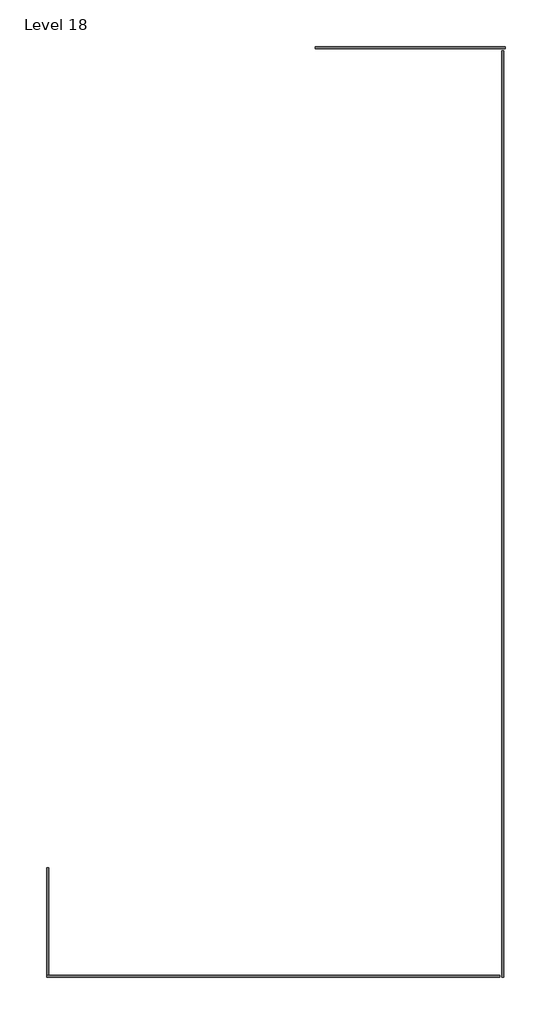
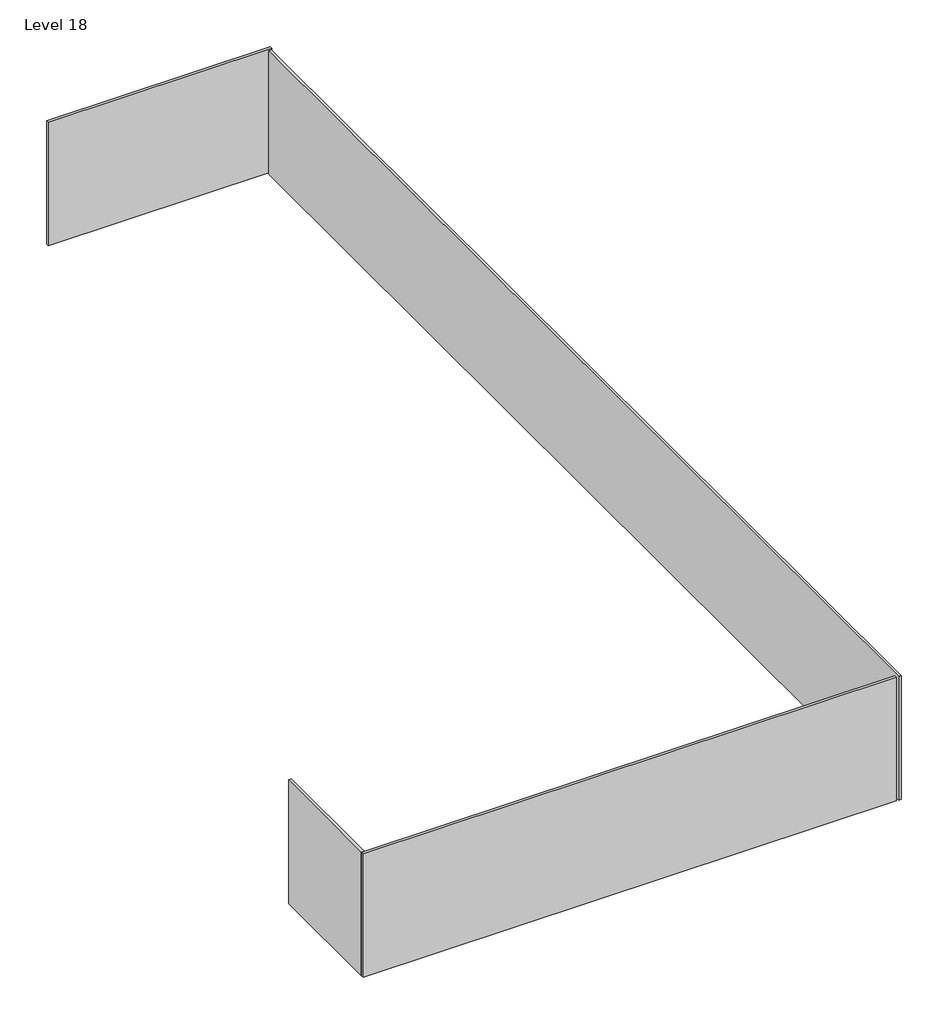
# One storey: 4 plates.
"""IFC4 building model written with IfcOpenShell, lengths in millimetres."""

from ifc_helpers import new_model, si_unit, origin, place, context, project, spatial, transform, mapped, element, save
from components import system_panel_glazed_6865593f, system_panel_glazed_cbb493b5, system_panel_glazed_6393fe79, system_panel_glazed_6dbe1261

model = new_model("IFC4")

# Units and contexts
model_context = context("Model", 3, world=origin())
ifc_project = project(units=[si_unit("LENGTHUNIT", "METRE", prefix="MILLI")], contexts=[model_context])

# Site, building, storey
site = spatial("IfcSite", under=ifc_project)
building = spatial("IfcBuilding", under=site)
storey = spatial("IfcBuildingStorey", under=building, Name="Level 18", Elevation=29260.8)

# Plates
placement = place(None, origin())
system_panel_glazed_shape = system_panel_glazed_6865593f(model_context)
element("IfcPlate", 1, ObjectType="System Panel : Glazed", at=placement, inside=storey, context=model_context, shape_type="MappedRepresentation", body=[
    mapped(system_panel_glazed_shape, transform((9033.0791312, -5892.9308221, 29260.8), x_axis=(1.0, 0.0, 0.0), y_axis=(0.0, 1.0, 0.0), z_axis=(0.0, 0.0, 1.0))),
])
system_panel_glazed_2_shape = system_panel_glazed_cbb493b5(model_context)
element("IfcPlate", 2, ObjectType="System Panel : Glazed", at=placement, inside=storey, context=model_context, shape_type="MappedRepresentation", body=[
    mapped(system_panel_glazed_2_shape, transform((10016.0464352, -10976.1058221, 29260.8), x_axis=(0.0, -1.0, 0.0), y_axis=(1.0, 0.0, 0.0), z_axis=(0.0, 0.0, 1.0))),
])
system_panel_glazed_3_shape = system_panel_glazed_6393fe79(model_context)
element("IfcPlate", 3, ObjectType="System Panel : Glazed", at=placement, inside=storey, context=model_context, shape_type="MappedRepresentation", body=[
    mapped(system_panel_glazed_3_shape, transform((7531.3041312, -16014.8308221, 29260.8), x_axis=(-1.0, 0.0, 0.0), y_axis=(0.0, -1.0, 0.0), z_axis=(0.0, 0.0, 1.0))),
])
system_panel_glazed_4_shape = system_panel_glazed_6dbe1261(model_context)
element("IfcPlate", 4, ObjectType="System Panel : Glazed", at=placement, inside=storey, context=model_context, shape_type="MappedRepresentation", body=[
    mapped(system_panel_glazed_4_shape, transform((5088.4464352, -15446.0293258, 29260.8), x_axis=(0.0, 1.0, 0.0), y_axis=(-1.0, 0.0, 0.0), z_axis=(0.0, 0.0, 1.0))),
])

save(model, "model.ifc")

# Revit data of these elements
# Type "System Panel : Glazed"
#   Construction Type Id = "GSP4R"
#   Analytic Construction = "1/8 in Pilkington single glazing"
#   Visual Light Transmittance = 0.9
#   Solar Heat Gain Coefficient = 0.86
#   Heat Transfer Coefficient (U) = 1.18115 BTU/(h·ft²·°F)
# Elements 1, 2, 3, 4 (IfcPlate, "System Panel : Glazed")
#   Phase Created = New Construction
#   Materials on its faces: "Glass"
# Materials
#   "Glass": class "Glass", colour RGB 0 128 192, transparency 0.75, Description = "Soda Lime Glass", Cost = 0
